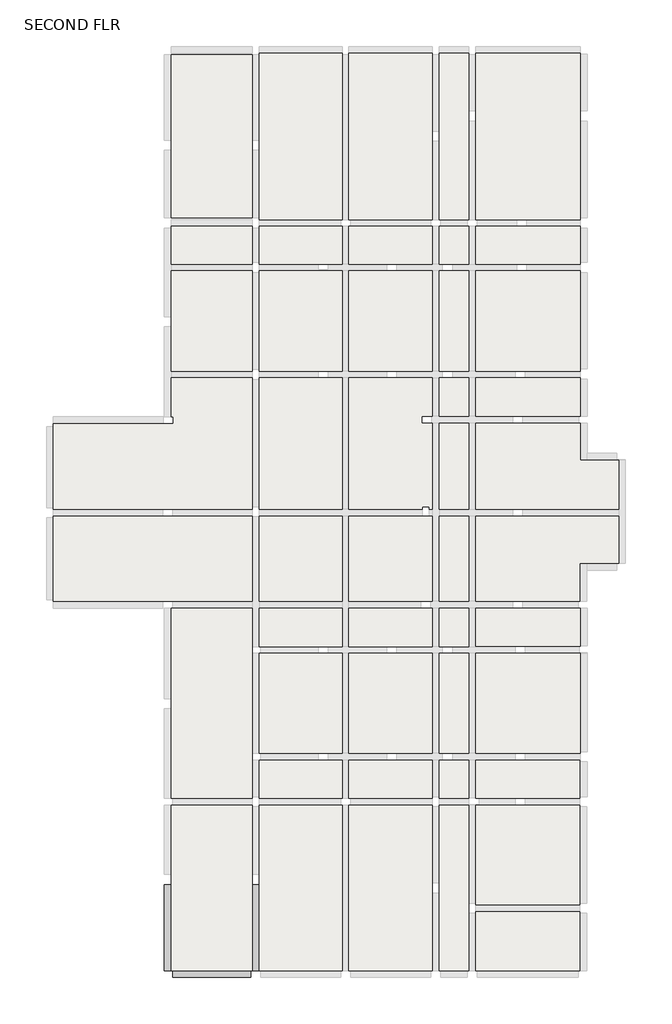
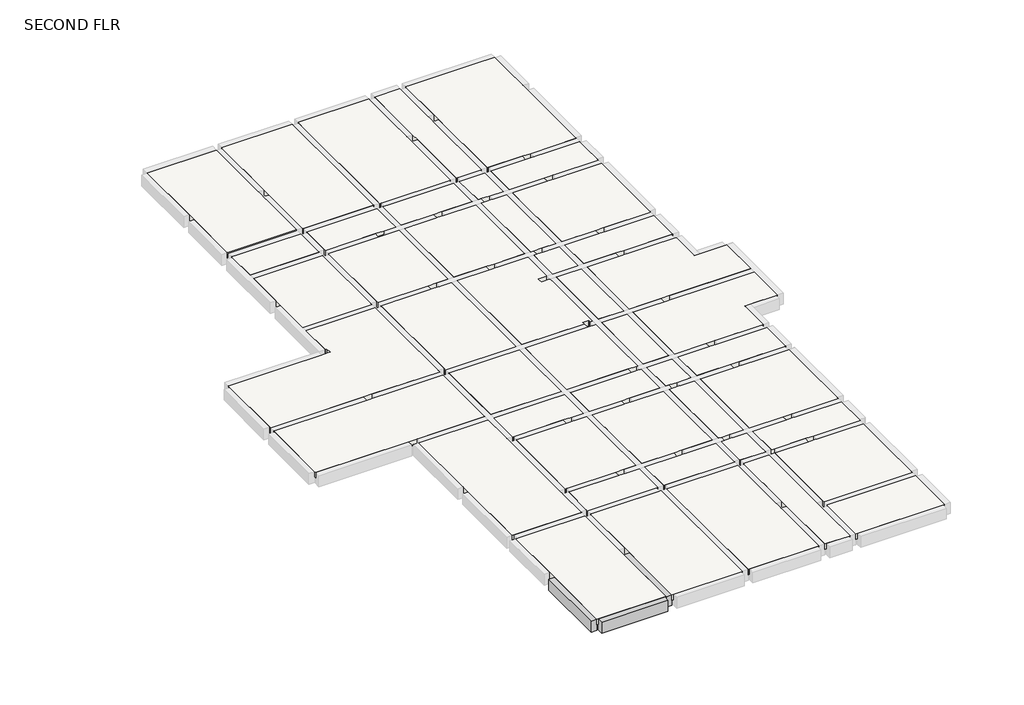
# One storey, part 1 of 4: 3 beams, 2 slabs.
"""IFC4 building model written with IfcOpenShell, lengths in millimetres."""

from ifc_helpers import new_model, si_unit, frame, origin, place, context, project, spatial, polyline, outline, extrude, faceted_brep, element, save

model = new_model("IFC4")

# Units and contexts
model_context = context("Model", 3, world=origin())
ifc_project = project(units=[si_unit("LENGTHUNIT", "METRE", prefix="MILLI")], contexts=[model_context])

# Site, building, storey
site = spatial("IfcSite", under=ifc_project)
building = spatial("IfcBuilding", under=site)
storey = spatial("IfcBuildingStorey", under=building, Name="SECOND FLR", Elevation=6048.0)

# Beams
placement = place(None, origin())
element("IfcBeam", 1, ObjectType="M_Concrete-Rectangular Beam : 300 x 600mm", at=placement, inside=storey, context=model_context, shape_type="Brep", body=[
    faceted_brep([(-5588.8105653, -15441.2517597, 6048.0), (-5888.8105653, -15441.2517597, 6048.0), (-5888.8105653, -19272.5304373, 6048.0), (-5588.8105653, -19272.5304373, 6048.0), (-5888.8105653, -15441.2517597, 5448.0), (-5888.8105653, -19272.5304373, 5448.0), (-5588.8105653, -15441.2517597, 5448.0), (-5588.8105653, -19272.5304373, 5448.0), (-5588.8105653, -19272.5304373, 5748.0), (-5588.8105653, -15441.2517597, 5748.0)], [[[0, 1, 2, 3]], [[1, 4, 5, 2]], [[4, 6, 7, 5]], [[0, 3, 8, 7, 6, 9]], [[6, 4, 1, 0, 9]], [[3, 2, 5, 7, 8]]]),
])
element("IfcBeam", 2, ObjectType="M_Concrete-Rectangular Beam : 300 x 600mm", at=placement, inside=storey, context=model_context, shape_type="SweptSolid", body=[
    extrude(outline(polyline([(-2046.7865686, -19272.5304373), (-2046.7865686, -19572.5304373), (-5516.7865686, -19572.5304373), (-5516.7865686, -19272.5304373), (-2046.7865686, -19272.5304373)])), frame((0.0, 0.0, 5448.0), z_axis=(0.0, 0.0, 1.0), x_axis=(1.0, 0.0, 0.0)), (0.0, 0.0, 1.0), 600.0),
])
element("IfcBeam", 3, ObjectType="M_Concrete-Rectangular Beam : 300 x 600mm", at=placement, inside=storey, context=model_context, shape_type="Brep", body=[
    faceted_brep([(-1971.7865686, -15441.2517597, 6048.0), (-1971.7865686, -19272.5304373, 6048.0), (-1671.7865686, -19272.5304373, 6048.0), (-1671.7865686, -15441.2517597, 6048.0), (-1671.7865686, -19272.5304373, 5748.0), (-1671.7865686, -19272.5304373, 5448.0), (-1671.7865686, -15441.2517597, 5448.0), (-1671.7865686, -15441.2517597, 5748.0), (-1971.7865686, -19272.5304373, 5448.0), (-1971.7865686, -15441.2517597, 5448.0), (-1971.7865686, -15441.2517597, 5748.0), (-1971.7865686, -19272.5304373, 5748.0)], [[[0, 1, 2, 3]], [[3, 2, 4, 5, 6, 7]], [[6, 5, 8, 9]], [[1, 0, 10, 9, 8, 11]], [[0, 3, 7, 6, 9, 10]], [[8, 5, 4, 2, 1, 11]]]),
])

# Slabs
element("IfcSlab", 4, ObjectType="Generic 300mm", at=placement, inside=storey, context=model_context, shape_type="Brep", body=[
    faceted_brep([(-1971.7865686, 21462.8349362, 5748.0), (-1971.7865686, 14212.5179708, 5748.0), (-5588.8105653, 14212.5179708, 5748.0), (-5591.7865686, 14212.5179708, 5748.0), (-5591.7865686, 17224.7148651, 5748.0), (-5591.7865686, 17674.7148651, 5748.0), (-5591.7865686, 21462.8349362, 5748.0), (-1971.7865686, 21462.8349362, 6048.0), (-5591.7865686, 21462.8349362, 6048.0), (-5591.7865686, 17674.7148651, 6048.0), (-5591.7865686, 17224.7148651, 6048.0), (-5591.7865686, 14212.5179708, 6048.0), (-5588.8105653, 14212.5179708, 6048.0), (-1971.7865686, 14212.5179708, 6048.0), (-1971.7865686, 17224.7148651, 6048.0), (-1971.7865686, 17674.7148651, 6048.0)], [[[0, 1, 2, 3, 4, 5, 6]], [[7, 8, 9, 10, 11, 12, 13, 14, 15]], [[1, 0, 7, 15, 14, 13]], [[3, 2, 1, 13, 12, 11]], [[6, 5, 4, 3, 11, 10, 9, 8]], [[0, 6, 8, 7]]]),
    faceted_brep([(2024.7296816, 21537.8349362, 5748.0), (2024.7296816, 14137.5179708, 5748.0), (-1671.7865686, 14137.5179708, 5748.0), (-1671.7865686, 21537.8349362, 5748.0), (2024.7296816, 21537.8349362, 6048.0), (-1671.7865686, 21537.8349362, 6048.0), (-1671.7865686, 21462.8349362, 6048.0), (-1671.7865686, 17674.7148651, 6048.0), (-1671.7865686, 17224.7148651, 6048.0), (-1671.7865686, 14212.5179708, 6048.0), (-1671.7865686, 14137.5179708, 6048.0), (1949.7296816, 14137.5179708, 6048.0), (2024.7296816, 14137.5179708, 6048.0), (2024.7296816, 21462.8349362, 6048.0)], [[[0, 1, 2, 3]], [[4, 5, 6, 7, 8, 9, 10, 11, 12, 13]], [[1, 0, 4, 13, 12]], [[2, 1, 12, 11, 10]], [[3, 2, 10, 9, 8, 7, 6, 5]], [[0, 3, 5, 4]]]),
    faceted_brep([(6032.5248054, 21537.8349362, 5748.0), (6032.5248054, 14137.5179708, 5748.0), (2324.7296816, 14137.5179708, 5748.0), (2324.7296816, 21537.8349362, 5748.0), (6032.5248054, 21537.8349362, 6048.0), (2324.7296816, 21537.8349362, 6048.0), (2324.7296816, 21462.8349362, 6048.0), (2324.7296816, 14137.5179708, 6048.0), (2399.7296816, 14137.5179708, 6048.0), (5957.5248054, 14137.5179708, 6048.0), (6032.5248054, 14137.5179708, 6048.0), (6032.5248054, 17624.7148651, 6048.0), (6032.5248054, 18074.7148651, 6048.0), (6032.5248054, 21462.8349362, 6048.0)], [[[0, 1, 2, 3]], [[4, 5, 6, 7, 8, 9, 10, 11, 12, 13]], [[1, 0, 4, 13, 12, 11, 10]], [[2, 1, 10, 9, 8, 7]], [[3, 2, 7, 6, 5]], [[0, 3, 5, 4]]]),
    faceted_brep([(7656.8679014, 21537.8349362, 5748.0), (7656.8679014, 14137.5179708, 5748.0), (6332.5248054, 14137.5179708, 5748.0), (6332.5248054, 21537.8349362, 5748.0), (7656.8679014, 21537.8349362, 6048.0), (6332.5248054, 21537.8349362, 6048.0), (6332.5248054, 21462.8349362, 6048.0), (6332.5248054, 18074.7148651, 6048.0), (6332.5248054, 17624.7148651, 6048.0), (6332.5248054, 14137.5179708, 6048.0), (6407.5248054, 14137.5179708, 6048.0), (7581.8679014, 14137.5179708, 6048.0), (7656.8679014, 14137.5179708, 6048.0), (7656.8679014, 18524.7148651, 6048.0), (7656.8679014, 18974.7148651, 6048.0), (7656.8679014, 21462.8349362, 6048.0)], [[[0, 1, 2, 3]], [[4, 5, 6, 7, 8, 9, 10, 11, 12, 13, 14, 15]], [[1, 0, 4, 15, 14, 13, 12]], [[2, 1, 12, 11, 10, 9]], [[3, 2, 9, 8, 7, 6, 5]], [[0, 3, 5, 4]]]),
    faceted_brep([(12619.1163908, 21537.8349362, 5748.0), (12619.1163908, 14137.5179708, 5748.0), (7956.8679014, 14137.5179708, 5748.0), (7956.8679014, 21537.8349362, 5748.0), (12619.1163908, 21537.8349362, 6048.0), (7956.8679014, 21537.8349362, 6048.0), (7956.8679014, 21462.8349362, 6048.0), (7956.8679014, 18974.7148651, 6048.0), (7956.8679014, 18524.7148651, 6048.0), (7956.8679014, 14137.5179708, 6048.0), (8031.8679014, 14137.5179708, 6048.0), (9781.8679014, 14137.5179708, 6048.0), (10231.8679014, 14137.5179708, 6048.0), (12619.1163908, 14137.5179708, 6048.0), (12619.1163908, 14212.5179708, 6048.0), (12619.1163908, 18524.7148651, 6048.0), (12619.1163908, 18974.7148651, 6048.0), (12619.1163908, 21502.8349362, 6048.0)], [[[0, 1, 2, 3]], [[4, 5, 6, 7, 8, 9, 10, 11, 12, 13, 14, 15, 16, 17]], [[1, 0, 4, 17, 16, 15, 14, 13]], [[2, 1, 13, 12, 11, 10, 9]], [[3, 2, 9, 8, 7, 6, 5]], [[0, 3, 5, 4]]]),
    faceted_brep([(-1971.7865686, 13837.5179708, 5748.0), (-1971.7865686, 12157.4075451, 5748.0), (-5588.8105653, 12157.4075451, 5748.0), (-5588.8105653, 13837.5179708, 5748.0), (-1971.7865686, 13837.5179708, 6048.0), (-5588.8105653, 13837.5179708, 6048.0), (-5588.8105653, 13762.5179708, 6048.0), (-5588.8105653, 12157.4075451, 6048.0), (-1971.7865686, 12157.4075451, 6048.0), (-1971.7865686, 12232.4075451, 6048.0), (-1971.7865686, 13762.5179708, 6048.0)], [[[0, 1, 2, 3]], [[4, 5, 6, 7, 8, 9, 10]], [[1, 0, 4, 10, 9, 8]], [[2, 1, 8, 7]], [[3, 2, 7, 6, 5]], [[0, 3, 5, 4]]]),
    faceted_brep([(2024.7296816, 13837.5179708, 5748.0), (2024.7296816, 12157.4075451, 5748.0), (1399.7296816, 12157.4075451, 5748.0), (949.7296816, 12157.4075451, 5748.0), (-1671.7865686, 12157.4075451, 5748.0), (-1671.7865686, 13837.5179708, 5748.0), (2024.7296816, 13837.5179708, 6048.0), (1949.7296816, 13837.5179708, 6048.0), (-1671.7865686, 13837.5179708, 6048.0), (-1671.7865686, 13762.5179708, 6048.0), (-1671.7865686, 12232.4075451, 6048.0), (-1671.7865686, 12157.4075451, 6048.0), (949.7296816, 12157.4075451, 6048.0), (1399.7296816, 12157.4075451, 6048.0), (2024.7296816, 12157.4075451, 6048.0)], [[[0, 1, 2, 3, 4, 5]], [[6, 7, 8, 9, 10, 11, 12, 13, 14]], [[1, 0, 6, 14]], [[4, 3, 2, 1, 14, 13, 12, 11]], [[5, 4, 11, 10, 9, 8]], [[0, 5, 8, 7, 6]]]),
    faceted_brep([(6032.5248054, 13837.5179708, 5748.0), (6032.5248054, 12157.4075451, 5748.0), (2324.7296816, 12157.4075451, 5748.0), (2324.7296816, 13837.5179708, 5748.0), (6032.5248054, 13837.5179708, 6048.0), (5957.5248054, 13837.5179708, 6048.0), (2399.7296816, 13837.5179708, 6048.0), (2324.7296816, 13837.5179708, 6048.0), (2324.7296816, 12157.4075451, 6048.0), (3997.5248054, 12157.4075451, 6048.0), (4447.5248054, 12157.4075451, 6048.0), (6032.5248054, 12157.4075451, 6048.0)], [[[0, 1, 2, 3]], [[4, 5, 6, 7, 8, 9, 10, 11]], [[1, 0, 4, 11]], [[2, 1, 11, 10, 9, 8]], [[3, 2, 8, 7]], [[0, 3, 7, 6, 5, 4]]]),
    faceted_brep([(7656.8679014, 13837.5179708, 5748.0), (7656.8679014, 12157.4075451, 5748.0), (6332.5248054, 12157.4075451, 5748.0), (6332.5248054, 13837.5179708, 5748.0), (7656.8679014, 13837.5179708, 6048.0), (7581.8679014, 13837.5179708, 6048.0), (6407.5248054, 13837.5179708, 6048.0), (6332.5248054, 13837.5179708, 6048.0), (6332.5248054, 12157.4075451, 6048.0), (6481.8679014, 12157.4075451, 6048.0), (6931.8679014, 12157.4075451, 6048.0), (7656.8679014, 12157.4075451, 6048.0)], [[[0, 1, 2, 3]], [[4, 5, 6, 7, 8, 9, 10, 11]], [[1, 0, 4, 11]], [[2, 1, 11, 10, 9, 8]], [[3, 2, 8, 7]], [[0, 3, 7, 6, 5, 4]]]),
    faceted_brep([(12619.1163908, 13837.5179708, 5748.0), (12619.1163908, 12157.4075451, 5748.0), (7956.8679014, 12157.4075451, 5748.0), (7956.8679014, 13837.5179708, 5748.0), (12619.1163908, 13837.5179708, 6048.0), (10231.8679014, 13837.5179708, 6048.0), (9781.8679014, 13837.5179708, 6048.0), (8031.8679014, 13837.5179708, 6048.0), (7956.8679014, 13837.5179708, 6048.0), (7956.8679014, 12157.4075451, 6048.0), (9781.8679014, 12157.4075451, 6048.0), (10231.8679014, 12157.4075451, 6048.0), (12619.1163908, 12157.4075451, 6048.0), (12619.1163908, 12232.4075451, 6048.0), (12619.1163908, 13762.5179708, 6048.0)], [[[0, 1, 2, 3]], [[4, 5, 6, 7, 8, 9, 10, 11, 12, 13, 14]], [[1, 0, 4, 14, 13, 12]], [[2, 1, 12, 11, 10, 9]], [[3, 2, 9, 8]], [[0, 3, 8, 7, 6, 5, 4]]]),
    faceted_brep([(-1971.7865686, 11857.4075451, 5748.0), (-1971.7865686, 7399.7076276, 5748.0), (-5588.8105653, 7399.7076276, 5748.0), (-5588.8105653, 11857.4075451, 5748.0), (-1971.7865686, 11857.4075451, 6048.0), (-5588.8105653, 11857.4075451, 6048.0), (-5588.8105653, 9817.5252033, 6048.0), (-5588.8105653, 9367.5252033, 6048.0), (-5588.8105653, 7399.7076276, 6048.0), (-1971.7865686, 7399.7076276, 6048.0), (-1971.7865686, 7474.7076276, 6048.0), (-1971.7865686, 11782.4075451, 6048.0)], [[[0, 1, 2, 3]], [[4, 5, 6, 7, 8, 9, 10, 11]], [[1, 0, 4, 11, 10, 9]], [[2, 1, 9, 8]], [[3, 2, 8, 7, 6, 5]], [[0, 3, 5, 4]]]),
    faceted_brep([(2024.7296816, 11857.4075451, 5748.0), (2024.7296816, 7399.7076276, 5748.0), (-1671.7865686, 7399.7076276, 5748.0), (-1671.7865686, 11857.4075451, 5748.0), (2024.7296816, 11857.4075451, 6048.0), (-1671.7865686, 11857.4075451, 6048.0), (-1671.7865686, 11782.4075451, 6048.0), (-1671.7865686, 7474.7076276, 6048.0), (-1671.7865686, 7399.7076276, 6048.0), (949.7296816, 7399.7076276, 6048.0), (1399.7296816, 7399.7076276, 6048.0), (2024.7296816, 7399.7076276, 6048.0)], [[[0, 1, 2, 3]], [[4, 5, 6, 7, 8, 9, 10, 11]], [[1, 0, 4, 11]], [[2, 1, 11, 10, 9, 8]], [[3, 2, 8, 7, 6, 5]], [[0, 3, 5, 4]]]),
    faceted_brep([(6032.5248054, 11857.4075451, 5748.0), (6032.5248054, 7399.7076276, 5748.0), (2324.7296816, 7399.7076276, 5748.0), (2324.7296816, 11857.4075451, 5748.0), (6032.5248054, 11857.4075451, 6048.0), (4447.5248054, 11857.4075451, 6048.0), (3997.5248054, 11857.4075451, 6048.0), (2324.7296816, 11857.4075451, 6048.0), (2324.7296816, 7399.7076276, 6048.0), (3997.5248054, 7399.7076276, 6048.0), (4447.5248054, 7399.7076276, 6048.0), (6032.5248054, 7399.7076276, 6048.0)], [[[0, 1, 2, 3]], [[4, 5, 6, 7, 8, 9, 10, 11]], [[1, 0, 4, 11]], [[2, 1, 11, 10, 9, 8]], [[3, 2, 8, 7]], [[0, 3, 7, 6, 5, 4]]]),
    faceted_brep([(7656.8679014, 11857.4075451, 5748.0), (7656.8679014, 7399.7076276, 5748.0), (6332.5248054, 7399.7076276, 5748.0), (6332.5248054, 11857.4075451, 5748.0), (7656.8679014, 11857.4075451, 6048.0), (6931.8679014, 11857.4075451, 6048.0), (6481.8679014, 11857.4075451, 6048.0), (6332.5248054, 11857.4075451, 6048.0), (6332.5248054, 7399.7076276, 6048.0), (6481.8679014, 7399.7076276, 6048.0), (6931.8679014, 7399.7076276, 6048.0), (7656.8679014, 7399.7076276, 6048.0)], [[[0, 1, 2, 3]], [[4, 5, 6, 7, 8, 9, 10, 11]], [[1, 0, 4, 11]], [[2, 1, 11, 10, 9, 8]], [[3, 2, 8, 7]], [[0, 3, 7, 6, 5, 4]]]),
    faceted_brep([(12616.8679014, 11857.4075451, 5748.0), (12616.8679014, 7399.7076276, 5748.0), (7956.8679014, 7399.7076276, 5748.0), (7956.8679014, 11857.4075451, 5748.0), (12616.8679014, 11857.4075451, 6048.0), (10231.8679014, 11857.4075451, 6048.0), (9781.8679014, 11857.4075451, 6048.0), (7956.8679014, 11857.4075451, 6048.0), (7956.8679014, 7399.7076276, 6048.0), (9721.8679014, 7399.7076276, 6048.0), (10171.8679014, 7399.7076276, 6048.0), (12616.8679014, 7399.7076276, 6048.0)], [[[0, 1, 2, 3]], [[4, 5, 6, 7, 8, 9, 10, 11]], [[1, 0, 4, 11]], [[2, 1, 11, 10, 9, 8]], [[3, 2, 8, 7]], [[0, 3, 7, 6, 5, 4]]]),
    faceted_brep([(7656.8679014, 7099.7076276, 5748.0), (7656.8679014, 5387.6057249, 5748.0), (6332.5248054, 5387.6057249, 5748.0), (6332.5248054, 7099.7076276, 5748.0), (7656.8679014, 7099.7076276, 6048.0), (6931.8679014, 7099.7076276, 6048.0), (6481.8679014, 7099.7076276, 6048.0), (6332.5248054, 7099.7076276, 6048.0), (6332.5248054, 5387.6057249, 6048.0), (7656.8679014, 5387.6057249, 6048.0)], [[[0, 1, 2, 3]], [[4, 5, 6, 7, 8, 9]], [[1, 0, 4, 9]], [[2, 1, 9, 8]], [[3, 2, 8, 7]], [[0, 3, 7, 6, 5, 4]]]),
    faceted_brep([(12616.8679014, 7099.7076276, 5748.0), (12616.8679014, 5387.6057249, 5748.0), (7956.8679014, 5387.6057249, 5748.0), (7956.8679014, 7099.7076276, 5748.0), (12616.8679014, 7099.7076276, 6048.0), (10171.8679014, 7099.7076276, 6048.0), (9721.8679014, 7099.7076276, 6048.0), (7956.8679014, 7099.7076276, 6048.0), (7956.8679014, 5387.6057249, 6048.0), (9601.8679014, 5387.6057249, 6048.0), (10051.8679014, 5387.6057249, 6048.0), (12541.8679014, 5387.6057249, 6048.0), (12616.8679014, 5387.6057249, 6048.0)], [[[0, 1, 2, 3]], [[4, 5, 6, 7, 8, 9, 10, 11, 12]], [[1, 0, 4, 12]], [[2, 1, 12, 11, 10, 9, 8]], [[3, 2, 8, 7]], [[0, 3, 7, 6, 5, 4]]]),
    faceted_brep([(7656.8679014, 5087.6057249, 5748.0), (7656.8679014, 1251.1713929, 5748.0), (6332.5248054, 1251.1713929, 5748.0), (6332.5248054, 5087.6057249, 5748.0), (7656.8679014, 5087.6057249, 6048.0), (6332.5248054, 5087.6057249, 6048.0), (6332.5248054, 1251.1713929, 6048.0), (7656.8679014, 1251.1713929, 6048.0)], [[[0, 1, 2, 3]], [[4, 5, 6, 7]], [[1, 0, 4, 7]], [[2, 1, 7, 6]], [[3, 2, 6, 5]], [[0, 3, 5, 4]]]),
    faceted_brep([(14319.1163908, 1251.1713929, 5748.0), (7956.8679014, 1251.1713929, 5748.0), (7956.8679014, 5087.6057249, 5748.0), (12616.8679014, 5087.6057249, 5748.0), (12616.8679014, 3435.7536525, 5748.0), (14319.1163908, 3435.7536525, 5748.0), (14319.1163908, 1251.1713929, 6048.0), (14319.1163908, 3435.7536525, 6048.0), (12916.8679014, 3435.7536525, 6048.0), (12616.8679014, 3435.7536525, 6048.0), (12616.8679014, 5087.6057249, 6048.0), (12541.8679014, 5087.6057249, 6048.0), (10051.8679014, 5087.6057249, 6048.0), (9601.8679014, 5087.6057249, 6048.0), (7956.8679014, 5087.6057249, 6048.0), (7956.8679014, 1251.1713929, 6048.0), (9601.8679014, 1251.1713929, 6048.0), (10051.8679014, 1251.1713929, 6048.0)], [[[0, 1, 2, 3, 4, 5]], [[6, 7, 8, 9, 10, 11, 12, 13, 14, 15, 16, 17]], [[1, 0, 6, 17, 16, 15]], [[2, 1, 15, 14]], [[3, 2, 14, 13, 12, 11, 10]], [[4, 3, 10, 9]], [[5, 4, 9, 8, 7]], [[0, 5, 7, 6]]]),
    faceted_brep([(7956.8679014, -2839.4535766, 5748.0), (7956.8679014, 951.1713929, 5748.0), (14319.1163908, 951.1713929, 5748.0), (14319.1163908, -1148.8286071, 5748.0), (12599.1163908, -1148.8286071, 5748.0), (12599.1163908, -2839.4535766, 5748.0), (7956.8679014, -2839.4535766, 6048.0), (9601.8679014, -2839.4535766, 6048.0), (10051.8679014, -2839.4535766, 6048.0), (12524.1163908, -2839.4535766, 6048.0), (12599.1163908, -2839.4535766, 6048.0), (12599.1163908, -1148.8286071, 6048.0), (12899.1163908, -1148.8286071, 6048.0), (14244.1163908, -1148.8286071, 6048.0), (14319.1163908, -1148.8286071, 6048.0), (14319.1163908, 951.1713929, 6048.0), (10051.8679014, 951.1713929, 6048.0), (9601.8679014, 951.1713929, 6048.0), (7956.8679014, 951.1713929, 6048.0)], [[[0, 1, 2, 3, 4, 5]], [[6, 7, 8, 9, 10, 11, 12, 13, 14, 15, 16, 17, 18]], [[1, 0, 6, 18]], [[2, 1, 18, 17, 16, 15]], [[3, 2, 15, 14]], [[4, 3, 14, 13, 12, 11]], [[5, 4, 11, 10]], [[0, 5, 10, 9, 8, 7, 6]]]),
    faceted_brep([(7656.8679014, 951.1713929, 5748.0), (7656.8679014, -2839.4535766, 5748.0), (6332.5248054, -2839.4535766, 5748.0), (6332.5248054, 951.1713929, 5748.0), (7656.8679014, 951.1713929, 6048.0), (6332.5248054, 951.1713929, 6048.0), (6332.5248054, -2839.4535766, 6048.0), (7656.8679014, -2839.4535766, 6048.0)], [[[0, 1, 2, 3]], [[4, 5, 6, 7]], [[1, 0, 4, 7]], [[2, 1, 7, 6]], [[3, 2, 6, 5]], [[0, 3, 5, 4]]]),
    faceted_brep([(6032.5248054, 951.1713929, 5748.0), (6032.5248054, -2839.4535766, 5748.0), (2324.7296816, -2839.4535766, 5748.0), (2324.7296816, 951.1713929, 5748.0), (5592.5248054, 951.1713929, 5748.0), (5892.5248054, 951.1713929, 5748.0), (6032.5248054, 951.1713929, 6048.0), (5892.5248054, 951.1713929, 6048.0), (5592.5248054, 951.1713929, 6048.0), (2324.7296816, 951.1713929, 6048.0), (2324.7296816, -2839.4535766, 6048.0), (5517.5248054, -2839.4535766, 6048.0), (5967.5248054, -2839.4535766, 6048.0), (6032.5248054, -2839.4535766, 6048.0)], [[[0, 1, 2, 3, 4, 5]], [[6, 7, 8, 9, 10, 11, 12, 13]], [[1, 0, 6, 13]], [[2, 1, 13, 12, 11, 10]], [[3, 2, 10, 9]], [[0, 5, 4, 3, 9, 8, 7, 6]]]),
    faceted_brep([(2024.7296816, 951.1713929, 5748.0), (2024.7296816, -2839.4535766, 5748.0), (-1671.7865686, -2839.4535766, 5748.0), (-1671.7865686, 951.1713929, 5748.0), (2024.7296816, 951.1713929, 6048.0), (-1671.7865686, 951.1713929, 6048.0), (-1671.7865686, 916.1713929, 6048.0), (-1671.7865686, -2839.4535766, 6048.0), (2024.7296816, -2839.4535766, 6048.0)], [[[0, 1, 2, 3]], [[4, 5, 6, 7, 8]], [[1, 0, 4, 8]], [[2, 1, 8, 7]], [[3, 2, 7, 6, 5]], [[0, 3, 5, 4]]]),
    faceted_brep([(2024.7296816, 7099.7076276, 5748.0), (2024.7296816, 1251.1713929, 5748.0), (-1671.7865686, 1251.1713929, 5748.0), (-1671.7865686, 7099.7076276, 5748.0), (2024.7296816, 7099.7076276, 6048.0), (1399.7296816, 7099.7076276, 6048.0), (949.7296816, 7099.7076276, 6048.0), (-1671.7865686, 7099.7076276, 6048.0), (-1671.7865686, 7024.7076276, 6048.0), (-1671.7865686, 1366.1713929, 6048.0), (-1671.7865686, 1251.1713929, 6048.0), (2024.7296816, 1251.1713929, 6048.0)], [[[0, 1, 2, 3]], [[4, 5, 6, 7, 8, 9, 10, 11]], [[1, 0, 4, 11]], [[2, 1, 11, 10]], [[3, 2, 10, 9, 8, 7]], [[0, 3, 7, 6, 5, 4]]]),
    faceted_brep([(-10828.8105653, 1251.1713929, 5748.0), (-10828.8105653, 5067.6057249, 5748.0), (-5493.8105653, 5067.6057249, 5748.0), (-5493.8105653, 5367.5252033, 5748.0), (-5588.8105653, 5367.5252033, 5748.0), (-5588.8105653, 7099.7076276, 5748.0), (-1971.7865686, 7099.7076276, 5748.0), (-1971.7865686, 1251.1713929, 5748.0), (-10828.8105653, 1251.1713929, 6048.0), (-5963.8105653, 1251.1713929, 6048.0), (-5513.8105653, 1251.1713929, 6048.0), (-1971.7865686, 1251.1713929, 6048.0), (-1971.7865686, 1366.1713929, 6048.0), (-1971.7865686, 7024.7076276, 6048.0), (-1971.7865686, 7099.7076276, 6048.0), (-5588.8105653, 7099.7076276, 6048.0), (-5588.8105653, 5367.5252033, 6048.0), (-5493.8105653, 5367.5252033, 6048.0), (-5493.8105653, 5067.6057249, 6048.0), (-5943.8105653, 5067.6057249, 6048.0), (-10828.8105653, 5067.6057249, 6048.0), (-10828.8105653, 4932.6057249, 6048.0), (-10828.8105653, 1326.1713929, 6048.0)], [[[0, 1, 2, 3, 4, 5, 6, 7]], [[8, 9, 10, 11, 12, 13, 14, 15, 16, 17, 18, 19, 20, 21, 22]], [[1, 0, 8, 22, 21, 20]], [[2, 1, 20, 19, 18]], [[3, 2, 18, 17]], [[4, 3, 17, 16]], [[5, 4, 16, 15]], [[6, 5, 15, 14]], [[7, 6, 14, 13, 12, 11]], [[0, 7, 11, 10, 9, 8]]]),
    faceted_brep([(-1971.7865686, -2839.4535766, 5748.0), (-10828.8105653, -2839.4535766, 5748.0), (-10828.8105653, 951.1713929, 5748.0), (-1971.7865686, 951.1713929, 5748.0), (-1971.7865686, -2839.4535766, 6048.0), (-1971.7865686, 916.1713929, 6048.0), (-1971.7865686, 951.1713929, 6048.0), (-5513.8105653, 951.1713929, 6048.0), (-5963.8105653, 951.1713929, 6048.0), (-10828.8105653, 951.1713929, 6048.0), (-10828.8105653, 876.1713929, 6048.0), (-10828.8105653, -2764.4535766, 6048.0), (-10828.8105653, -2839.4535766, 6048.0), (-5963.8105653, -2839.4535766, 6048.0), (-5513.8105653, -2839.4535766, 6048.0)], [[[0, 1, 2, 3]], [[4, 5, 6, 7, 8, 9, 10, 11, 12, 13, 14]], [[1, 0, 4, 14, 13, 12]], [[2, 1, 12, 11, 10, 9]], [[3, 2, 9, 8, 7, 6]], [[0, 3, 6, 5, 4]]]),
    faceted_brep([(2024.7296816, -3139.4535766, 5748.0), (2024.7296816, -4851.6229916, 5748.0), (-1671.7865686, -4851.6229916, 5748.0), (-1671.7865686, -3139.4535766, 5748.0), (2024.7296816, -3139.4535766, 6048.0), (-1671.7865686, -3139.4535766, 6048.0), (-1671.7865686, -4851.6229916, 6048.0), (-1596.7865686, -4851.6229916, 6048.0), (949.7296816, -4851.6229916, 6048.0), (1399.7296816, -4851.6229916, 6048.0), (2024.7296816, -4851.6229916, 6048.0)], [[[0, 1, 2, 3]], [[4, 5, 6, 7, 8, 9, 10]], [[1, 0, 4, 10]], [[2, 1, 10, 9, 8, 7, 6]], [[3, 2, 6, 5]], [[0, 3, 5, 4]]]),
    faceted_brep([(6032.5248054, -3139.4535766, 5748.0), (6032.5248054, -4851.6229916, 5748.0), (2324.7296816, -4851.6229916, 5748.0), (2324.7296816, -3139.4535766, 5748.0), (6032.5248054, -3139.4535766, 6048.0), (5967.5248054, -3139.4535766, 6048.0), (5517.5248054, -3139.4535766, 6048.0), (2324.7296816, -3139.4535766, 6048.0), (2324.7296816, -4851.6229916, 6048.0), (3997.5248054, -4851.6229916, 6048.0), (4447.5248054, -4851.6229916, 6048.0), (6032.5248054, -4851.6229916, 6048.0)], [[[0, 1, 2, 3]], [[4, 5, 6, 7, 8, 9, 10, 11]], [[1, 0, 4, 11]], [[2, 1, 11, 10, 9, 8]], [[3, 2, 8, 7]], [[0, 3, 7, 6, 5, 4]]]),
    faceted_brep([(2024.7296816, -5151.6229916, 5748.0), (2024.7296816, -9607.1078267, 5748.0), (-1671.7865686, -9607.1078267, 5748.0), (-1671.7865686, -5151.6229916, 5748.0), (2024.7296816, -5151.6229916, 6048.0), (1399.7296816, -5151.6229916, 6048.0), (949.7296816, -5151.6229916, 6048.0), (-1596.7865686, -5151.6229916, 6048.0), (-1671.7865686, -5151.6229916, 6048.0), (-1671.7865686, -9607.1078267, 6048.0), (-1596.7865686, -9607.1078267, 6048.0), (949.7296816, -9607.1078267, 6048.0), (1399.7296816, -9607.1078267, 6048.0), (2024.7296816, -9607.1078267, 6048.0)], [[[0, 1, 2, 3]], [[4, 5, 6, 7, 8, 9, 10, 11, 12, 13]], [[1, 0, 4, 13]], [[2, 1, 13, 12, 11, 10, 9]], [[3, 2, 9, 8]], [[0, 3, 8, 7, 6, 5, 4]]]),
    faceted_brep([(6032.5248054, -5151.6229916, 5748.0), (6032.5248054, -9607.1078267, 5748.0), (2324.7296816, -9607.1078267, 5748.0), (2324.7296816, -5151.6229916, 5748.0), (6032.5248054, -5151.6229916, 6048.0), (4447.5248054, -5151.6229916, 6048.0), (3997.5248054, -5151.6229916, 6048.0), (2324.7296816, -5151.6229916, 6048.0), (2324.7296816, -9607.1078267, 6048.0), (3997.5248054, -9607.1078267, 6048.0), (4447.5248054, -9607.1078267, 6048.0), (6032.5248054, -9607.1078267, 6048.0)], [[[0, 1, 2, 3]], [[4, 5, 6, 7, 8, 9, 10, 11]], [[1, 0, 4, 11]], [[2, 1, 11, 10, 9, 8]], [[3, 2, 8, 7]], [[0, 3, 7, 6, 5, 4]]]),
    faceted_brep([(7656.8679014, -5151.6229916, 5748.0), (7656.8679014, -9607.1078267, 5748.0), (6332.5248054, -9607.1078267, 5748.0), (6332.5248054, -5151.6229916, 5748.0), (7656.8679014, -5151.6229916, 6048.0), (6931.8679014, -5151.6229916, 6048.0), (6481.8679014, -5151.6229916, 6048.0), (6332.5248054, -5151.6229916, 6048.0), (6332.5248054, -9607.1078267, 6048.0), (6481.8679014, -9607.1078267, 6048.0), (6931.8679014, -9607.1078267, 6048.0), (7656.8679014, -9607.1078267, 6048.0)], [[[0, 1, 2, 3]], [[4, 5, 6, 7, 8, 9, 10, 11]], [[1, 0, 4, 11]], [[2, 1, 11, 10, 9, 8]], [[3, 2, 8, 7]], [[0, 3, 7, 6, 5, 4]]]),
    faceted_brep([(12619.1163908, -3139.4535766, 5748.0), (12619.1163908, -4831.6229916, 5748.0), (7956.8679014, -4831.6229916, 5748.0), (7956.8679014, -3139.4535766, 5748.0), (12619.1163908, -3139.4535766, 6048.0), (12524.1163908, -3139.4535766, 6048.0), (10051.8679014, -3139.4535766, 6048.0), (9601.8679014, -3139.4535766, 6048.0), (7956.8679014, -3139.4535766, 6048.0), (7956.8679014, -4831.6229916, 6048.0), (12564.1163908, -4831.6229916, 6048.0), (12619.1163908, -4831.6229916, 6048.0), (12619.1163908, -4818.9229916, 6048.0)], [[[0, 1, 2, 3]], [[4, 5, 6, 7, 8, 9, 10, 11, 12]], [[1, 0, 4, 12, 11]], [[2, 1, 11, 10, 9]], [[3, 2, 9, 8]], [[0, 3, 8, 7, 6, 5, 4]]]),
    faceted_brep([(12619.1163908, -5151.6229916, 5748.0), (12619.1163908, -9607.1078267, 5748.0), (7956.8679014, -9607.1078267, 5748.0), (7956.8679014, -5151.6229916, 5748.0), (12619.1163908, -5151.6229916, 6048.0), (10171.8679014, -5151.6229916, 6048.0), (9721.8679014, -5151.6229916, 6048.0), (7956.8679014, -5151.6229916, 6048.0), (7956.8679014, -9607.1078267, 6048.0), (9721.8679014, -9607.1078267, 6048.0), (10171.8679014, -9607.1078267, 6048.0), (12619.1163908, -9607.1078267, 6048.0), (12619.1163908, -9532.1078267, 6048.0)], [[[0, 1, 2, 3]], [[4, 5, 6, 7, 8, 9, 10, 11, 12]], [[1, 0, 4, 12, 11]], [[2, 1, 11, 10, 9, 8]], [[3, 2, 8, 7]], [[0, 3, 7, 6, 5, 4]]]),
    faceted_brep([(12599.1163908, -9907.1078267, 5748.0), (12599.1163908, -11607.8970059, 5748.0), (8111.8679014, -11607.8970059, 5748.0), (7956.8679014, -11607.8970059, 5748.0), (7956.8679014, -11587.8970059, 5748.0), (7956.8679014, -9907.1078267, 5748.0), (12599.1163908, -9907.1078267, 6048.0), (10171.8679014, -9907.1078267, 6048.0), (9721.8679014, -9907.1078267, 6048.0), (7956.8679014, -9907.1078267, 6048.0), (7956.8679014, -11587.8970059, 6048.0), (7956.8679014, -11607.8970059, 6048.0), (8111.8679014, -11607.8970059, 6048.0), (9721.8679014, -11607.8970059, 6048.0), (10171.8679014, -11607.8970059, 6048.0), (12599.1163908, -11607.8970059, 6048.0), (12599.1163908, -11532.8970059, 6048.0)], [[[0, 1, 2, 3, 4, 5]], [[6, 7, 8, 9, 10, 11, 12, 13, 14, 15, 16]], [[1, 0, 6, 16, 15]], [[3, 2, 1, 15, 14, 13, 12, 11]], [[5, 4, 3, 11, 10, 9]], [[0, 5, 9, 8, 7, 6]]]),
    faceted_brep([(7656.8679014, -9907.1078267, 5748.0), (7656.8679014, -11607.8970059, 5748.0), (6332.5248054, -11607.8970059, 5748.0), (6332.5248054, -9907.1078267, 5748.0), (7656.8679014, -9907.1078267, 6048.0), (6931.8679014, -9907.1078267, 6048.0), (6481.8679014, -9907.1078267, 6048.0), (6332.5248054, -9907.1078267, 6048.0), (6332.5248054, -11532.8970059, 6048.0), (6332.5248054, -11607.8970059, 6048.0), (7656.8679014, -11607.8970059, 6048.0)], [[[0, 1, 2, 3]], [[4, 5, 6, 7, 8, 9, 10]], [[1, 0, 4, 10]], [[2, 1, 10, 9]], [[3, 2, 9, 8, 7]], [[0, 3, 7, 6, 5, 4]]]),
    faceted_brep([(6032.5248054, -9907.1078267, 5748.0), (6032.5248054, -11607.8970059, 5748.0), (2324.7296816, -11607.8970059, 5748.0), (2324.7296816, -9907.1078267, 5748.0), (6032.5248054, -9907.1078267, 6048.0), (4447.5248054, -9907.1078267, 6048.0), (3997.5248054, -9907.1078267, 6048.0), (2324.7296816, -9907.1078267, 6048.0), (2324.7296816, -11607.8970059, 6048.0), (2399.7296816, -11607.8970059, 6048.0), (6032.5248054, -11607.8970059, 6048.0), (6032.5248054, -11532.8970059, 6048.0)], [[[0, 1, 2, 3]], [[4, 5, 6, 7, 8, 9, 10, 11]], [[1, 0, 4, 11, 10]], [[2, 1, 10, 9, 8]], [[3, 2, 8, 7]], [[0, 3, 7, 6, 5, 4]]]),
    faceted_brep([(2024.7296816, -9907.1078267, 5748.0), (2024.7296816, -11607.8970059, 5748.0), (-1671.7865686, -11607.8970059, 5748.0), (-1671.7865686, -9907.1078267, 5748.0), (2024.7296816, -9907.1078267, 6048.0), (1399.7296816, -9907.1078267, 6048.0), (949.7296816, -9907.1078267, 6048.0), (-1596.7865686, -9907.1078267, 6048.0), (-1671.7865686, -9907.1078267, 6048.0), (-1671.7865686, -11532.8970059, 6048.0), (-1671.7865686, -11607.8970059, 6048.0), (1949.7296816, -11607.8970059, 6048.0), (2024.7296816, -11607.8970059, 6048.0)], [[[0, 1, 2, 3]], [[4, 5, 6, 7, 8, 9, 10, 11, 12]], [[1, 0, 4, 12]], [[2, 1, 12, 11, 10]], [[3, 2, 10, 9, 8]], [[0, 3, 8, 7, 6, 5, 4]]]),
    faceted_brep([(2024.7296816, -11907.8970059, 5748.0), (2024.7296816, -19272.5304373, 5748.0), (-1671.7865686, -19272.5304373, 5748.0), (-1671.7865686, -11907.8970059, 5748.0), (2024.7296816, -11907.8970059, 6048.0), (1949.7296816, -11907.8970059, 6048.0), (-1671.7865686, -11907.8970059, 6048.0), (-1671.7865686, -11982.8970059, 6048.0), (-1671.7865686, -14991.2517597, 6048.0), (-1671.7865686, -15441.2517597, 6048.0), (-1671.7865686, -19272.5304373, 6048.0), (-1596.7865686, -19272.5304373, 6048.0), (1949.7296816, -19272.5304373, 6048.0), (2024.7296816, -19272.5304373, 6048.0)], [[[0, 1, 2, 3]], [[4, 5, 6, 7, 8, 9, 10, 11, 12, 13]], [[1, 0, 4, 13]], [[2, 1, 13, 12, 11, 10]], [[3, 2, 10, 9, 8, 7, 6]], [[0, 3, 6, 5, 4]]]),
    faceted_brep([(6032.5248054, -11907.8970059, 5748.0), (6032.5248054, -19272.5304373, 5748.0), (2324.7296816, -19272.5304373, 5748.0), (2324.7296816, -11907.8970059, 5748.0), (6032.5248054, -11907.8970059, 6048.0), (2399.7296816, -11907.8970059, 6048.0), (2324.7296816, -11907.8970059, 6048.0), (2324.7296816, -19272.5304373, 6048.0), (2399.7296816, -19272.5304373, 6048.0), (5957.5248054, -19272.5304373, 6048.0), (6032.5248054, -19272.5304373, 6048.0), (6032.5248054, -15819.1579597, 6048.0), (6032.5248054, -15369.1579597, 6048.0), (6032.5248054, -11982.8970059, 6048.0)], [[[0, 1, 2, 3]], [[4, 5, 6, 7, 8, 9, 10, 11, 12, 13]], [[1, 0, 4, 13, 12, 11, 10]], [[2, 1, 10, 9, 8, 7]], [[3, 2, 7, 6]], [[0, 3, 6, 5, 4]]]),
    faceted_brep([(7656.8679014, -11907.8970059, 5748.0), (7656.8679014, -19272.5304373, 5748.0), (6332.5248054, -19272.5304373, 5748.0), (6332.5248054, -11907.8970059, 5748.0), (7656.8679014, -11907.8970059, 6048.0), (6332.5248054, -11907.8970059, 6048.0), (6332.5248054, -11982.8970059, 6048.0), (6332.5248054, -15369.1579597, 6048.0), (6332.5248054, -15819.1579597, 6048.0), (6332.5248054, -19272.5304373, 6048.0), (6407.5248054, -19272.5304373, 6048.0), (7581.8679014, -19272.5304373, 6048.0), (7656.8679014, -19272.5304373, 6048.0), (7656.8679014, -16719.1579597, 6048.0), (7656.8679014, -16269.1579597, 6048.0)], [[[0, 1, 2, 3]], [[4, 5, 6, 7, 8, 9, 10, 11, 12, 13, 14]], [[1, 0, 4, 14, 13, 12]], [[2, 1, 12, 11, 10, 9]], [[3, 2, 9, 8, 7, 6, 5]], [[0, 3, 5, 4]]]),
    faceted_brep([(12599.1163908, -16644.1579597, 5748.0), (12599.1163908, -19272.5304373, 5748.0), (7956.8679014, -19272.5304373, 5748.0), (7956.8679014, -16644.1579597, 5748.0), (12599.1163908, -16644.1579597, 6048.0), (7956.8679014, -16644.1579597, 6048.0), (7956.8679014, -16719.1579597, 6048.0), (7956.8679014, -19272.5304373, 6048.0), (8031.8679014, -19272.5304373, 6048.0), (12524.1163908, -19272.5304373, 6048.0), (12599.1163908, -19272.5304373, 6048.0), (12599.1163908, -16719.1579597, 6048.0)], [[[0, 1, 2, 3]], [[4, 5, 6, 7, 8, 9, 10, 11]], [[1, 0, 4, 11, 10]], [[2, 1, 10, 9, 8, 7]], [[3, 2, 7, 6, 5]], [[0, 3, 5, 4]]]),
    faceted_brep([(12599.1163908, -11907.8970059, 5748.0), (12599.1163908, -16344.1579597, 5748.0), (7956.8679014, -16344.1579597, 5748.0), (7956.8679014, -11907.8970059, 5748.0), (12599.1163908, -11907.8970059, 6048.0), (10171.8679014, -11907.8970059, 6048.0), (9721.8679014, -11907.8970059, 6048.0), (7956.8679014, -11907.8970059, 6048.0), (7956.8679014, -16269.1579597, 6048.0), (7956.8679014, -16344.1579597, 6048.0), (12599.1163908, -16344.1579597, 6048.0), (12599.1163908, -16269.1579597, 6048.0), (12599.1163908, -11982.8970059, 6048.0)], [[[0, 1, 2, 3]], [[4, 5, 6, 7, 8, 9, 10, 11, 12]], [[1, 0, 4, 12, 11, 10]], [[2, 1, 10, 9]], [[3, 2, 9, 8, 7]], [[0, 3, 7, 6, 5, 4]]]),
    faceted_brep([(6032.5248054, 7099.7076276, 5748.0), (6032.5248054, 5387.6057249, 5748.0), (5557.5248054, 5387.6057249, 5748.0), (5557.5248054, 5087.6057249, 5748.0), (6032.5248054, 5087.6057249, 5748.0), (6032.5248054, 1251.1713929, 5748.0), (5892.5248054, 1251.1713929, 5748.0), (5892.5248054, 1366.1713929, 5748.0), (5592.5248054, 1366.1713929, 5748.0), (5592.5248054, 1251.1713929, 5748.0), (2324.7296816, 1251.1713929, 5748.0), (2324.7296816, 5087.6057249, 5748.0), (2324.7296816, 5387.6057249, 5748.0), (2324.7296816, 7099.7076276, 5748.0), (6032.5248054, 7099.7076276, 6048.0), (4447.5248054, 7099.7076276, 6048.0), (3997.5248054, 7099.7076276, 6048.0), (2324.7296816, 7099.7076276, 6048.0), (2324.7296816, 1251.1713929, 6048.0), (5592.5248054, 1251.1713929, 6048.0), (5592.5248054, 1366.1713929, 6048.0), (5892.5248054, 1366.1713929, 6048.0), (5892.5248054, 1251.1713929, 6048.0), (6032.5248054, 1251.1713929, 6048.0), (6032.5248054, 5087.6057249, 6048.0), (6007.5248054, 5087.6057249, 6048.0), (5557.5248054, 5087.6057249, 6048.0), (5557.5248054, 5387.6057249, 6048.0), (6007.5248054, 5387.6057249, 6048.0), (6032.5248054, 5387.6057249, 6048.0)], [[[0, 1, 2, 3, 4, 5, 6, 7, 8, 9, 10, 11, 12, 13]], [[14, 15, 16, 17, 18, 19, 20, 21, 22, 23, 24, 25, 26, 27, 28, 29]], [[1, 0, 14, 29]], [[2, 1, 29, 28, 27]], [[3, 2, 27, 26]], [[4, 3, 26, 25, 24]], [[5, 4, 24, 23]], [[6, 5, 23, 22]], [[7, 6, 22, 21]], [[8, 7, 21, 20]], [[9, 8, 20, 19]], [[10, 9, 19, 18]], [[13, 12, 11, 10, 18, 17]], [[0, 13, 17, 16, 15, 14]]]),
    faceted_brep([(-1971.7865686, -11907.8970059, 5748.0), (-1971.7865686, -19272.5304373, 5748.0), (-5588.8105653, -19272.5304373, 5748.0), (-5588.8105653, -11907.8970059, 5748.0), (-1971.7865686, -11907.8970059, 6048.0), (-5513.8105653, -11907.8970059, 6048.0), (-5588.8105653, -11907.8970059, 6048.0), (-5588.8105653, -14991.2517597, 6048.0), (-5588.8105653, -15441.2517597, 6048.0), (-5588.8105653, -19272.5304373, 6048.0), (-5516.7865686, -19272.5304373, 6048.0), (-2046.7865686, -19272.5304373, 6048.0), (-1971.7865686, -19272.5304373, 6048.0), (-1971.7865686, -15441.2517597, 6048.0), (-1971.7865686, -14991.2517597, 6048.0), (-1971.7865686, -11982.8970059, 6048.0)], [[[0, 1, 2, 3]], [[4, 5, 6, 7, 8, 9, 10, 11, 12, 13, 14, 15]], [[1, 0, 4, 15, 14, 13, 12]], [[2, 1, 12, 11, 10, 9]], [[3, 2, 9, 8, 7, 6]], [[0, 3, 6, 5, 4]]]),
    faceted_brep([(-1971.7865686, -3139.4535766, 5748.0), (-1971.7865686, -4851.6229916, 5748.0), (-1971.7865686, -5151.6229916, 5748.0), (-1971.7865686, -9607.1078267, 5748.0), (-1971.7865686, -9907.1078267, 5748.0), (-1971.7865686, -11607.8970059, 5748.0), (-5588.8105653, -11607.8970059, 5748.0), (-5588.8105653, -3139.4535766, 5748.0), (-1971.7865686, -3139.4535766, 6048.0), (-5513.8105653, -3139.4535766, 6048.0), (-5588.8105653, -3139.4535766, 6048.0), (-5588.8105653, -7169.0760584, 6048.0), (-5588.8105653, -7619.0760584, 6048.0), (-5588.8105653, -11607.8970059, 6048.0), (-5513.8105653, -11607.8970059, 6048.0), (-1971.7865686, -11607.8970059, 6048.0), (-1971.7865686, -11532.8970059, 6048.0), (-1971.7865686, -9907.1078267, 6048.0), (-1971.7865686, -9607.1078267, 6048.0), (-1971.7865686, -5151.6229916, 6048.0), (-1971.7865686, -4851.6229916, 6048.0)], [[[0, 1, 2, 3, 4, 5, 6, 7]], [[8, 9, 10, 11, 12, 13, 14, 15, 16, 17, 18, 19, 20]], [[5, 4, 3, 2, 1, 0, 8, 20, 19, 18, 17, 16, 15]], [[6, 5, 15, 14, 13]], [[7, 6, 13, 12, 11, 10]], [[0, 7, 10, 9, 8]]]),
])
element("IfcSlab", 5, ObjectType="Generic 300mm", at=placement, inside=storey, context=model_context, shape_type="Brep", body=[
    faceted_brep([(7656.8679014, -3139.4535766, 5748.0), (7656.8679014, -4851.6229916, 5748.0), (6332.5248054, -4851.6229916, 5748.0), (6332.5248054, -3139.4535766, 5748.0), (7656.8679014, -3139.4535766, 6048.0), (6332.5248054, -3139.4535766, 6048.0), (6332.5248054, -4851.6229916, 6048.0), (6481.8679014, -4851.6229916, 6048.0), (6931.8679014, -4851.6229916, 6048.0), (7656.8679014, -4851.6229916, 6048.0)], [[[0, 1, 2, 3]], [[4, 5, 6, 7, 8, 9]], [[1, 0, 4, 9]], [[2, 1, 9, 8, 7, 6]], [[3, 2, 6, 5]], [[0, 3, 5, 4]]]),
])

save(model, "model.ifc")

# Revit data of these elements
# Type "M_Concrete-Rectangular Beam : 300 x 600mm"
#   Length [instance default] = 1524 mm
#   b = 300 mm
#   h = 600 mm
#   Structural Material [instance default] = Concrete, Cast-in-Place gray
#   Assembly Code = ""
# Type "Generic 300mm"
#   Function = 0
#   Layers, outside or top first: 300 mm no material (function 1)
# Elements 1, 2, 3 (IfcBeam, "M_Concrete-Rectangular Beam : 300 x 600mm")
#   Structural Material = Concrete, Cast-in-Place gray
#   Phase Created = New Construction
#   Materials on its faces: "Concrete, Cast-in-Place gray"
# Elements 4, 5 (IfcSlab, "Generic 300mm")
#   Height Offset From Level = 0 mm
#   built-in parameter 1001954 = 1
#   Phase Created = New Construction
#   Materials on its faces: "Default Floor"
# Materials
#   "Concrete, Cast-in-Place gray": class "Concrete", colour RGB 192 192 192, transparency 0, Description = "Cast-in-place concrete", Cost = 0
#   "Default Floor": colour RGB 127 127 127, transparency 0, Cost = 0
